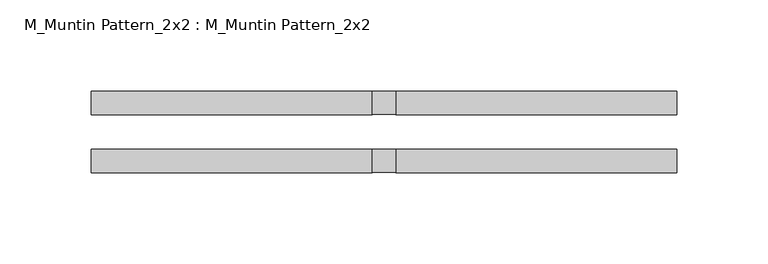
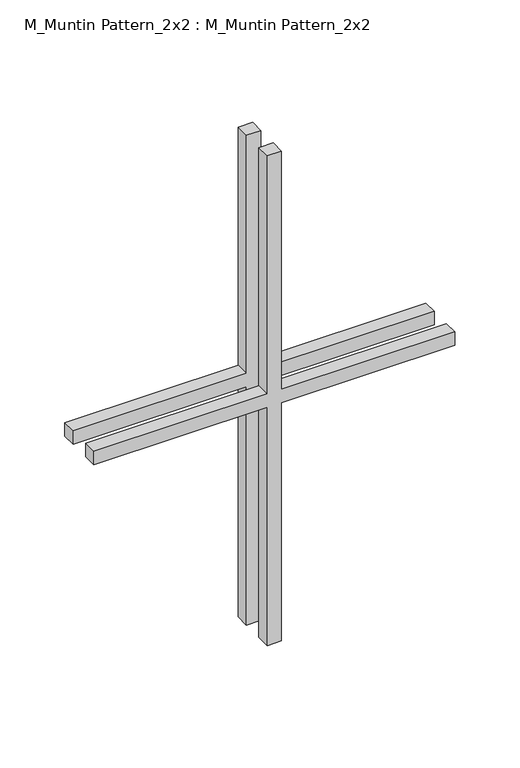
"""IFC4 building model written with IfcOpenShell, lengths in millimetres: proxy geometry, M_Muntin Pattern_2x2 : M_Muntin Pattern_2x2."""

from ifc_helpers import new_model, si_unit, frame, origin, place, context, project, spatial, polyline, outline, extrude, source, transform, mapped, element, save


def m_muntin_pattern_2x2_m_muntin_pattern_2x2_5c9fa27a(model_context):
    return source(origin(), model_context, "Body", "SweptSolid", [
        extrude(outline(polyline([(236.5, -6.35), (236.5, -160.3375), (223.8, -160.3375), (223.8, -6.35), (0.0, -6.35), (0.0, 6.35), (223.8, 6.35), (223.8, 160.3375), (236.5, 160.3375), (236.5, 6.35), (460.3, 6.35), (460.3, -6.35), (236.5, -6.35)])), frame((0.0, 9.525, 0.0), z_axis=(0.0, 1.0, 0.0), x_axis=(0.0, 0.0, 1.0)), (0.0, 0.0, 1.0), 12.7),
        extrude(outline(polyline([(236.5, -6.35), (236.5, -160.3375), (223.8, -160.3375), (223.8, -6.35), (0.0, -6.35), (0.0, 6.35), (223.8, 6.35), (223.8, 160.3375), (236.5, 160.3375), (236.5, 6.35), (460.3, 6.35), (460.3, -6.35), (236.5, -6.35)])), frame((0.0, -22.225, 0.0), z_axis=(0.0, 1.0, 0.0), x_axis=(0.0, 0.0, 1.0)), (0.0, 0.0, 1.0), 12.7),
    ])


if __name__ == "__main__":
    model = new_model("IFC4")
    model_context = context("Model", 3, world=origin())
    ifc_project = project(units=[si_unit("LENGTHUNIT", "METRE", prefix="MILLI")], contexts=[model_context])
    site = spatial("IfcSite", under=ifc_project)
    building = spatial("IfcBuilding", under=site)
    placement = place(None, origin())
    m_muntin_pattern_2x2_m_muntin_pattern_2x2_shape = m_muntin_pattern_2x2_m_muntin_pattern_2x2_5c9fa27a(model_context)
    element("IfcBuildingElementProxy", 1, Name="M_Muntin Pattern_2x2 : M_Muntin Pattern_2x2", ObjectType="M_Muntin Pattern_2x2 : M_Muntin Pattern_2x2", at=placement, inside=building, context=model_context, shape_type="MappedRepresentation", body=[
        mapped(m_muntin_pattern_2x2_m_muntin_pattern_2x2_shape, transform((0.0, 0.0, 0.0), x_axis=(1.0, 0.0, 0.0), y_axis=(0.0, 1.0, 0.0), z_axis=(0.0, 0.0, 1.0))),
    ])
    save(model, "model.ifc")

# Revit data of these elements
# Type "M_Muntin Pattern_2x2 : M_Muntin Pattern_2x2"
#   Width [instance default] = 3' - 11.24409"
#   Thickness = 0' - 0 1/2"
#   Height [instance default] = 3' - 11.24409"
#   Distance = 0' - 0 3/4"
#   Interior Material [instance default] = none
#   Exterior Material [instance default] = none
#   Default Elevation = 0
# Element 1 (IfcBuildingElementProxy, "M_Muntin Pattern_2x2 : M_Muntin Pattern_2x2")
#   Width = 1' - 0 5/8"
#   Height = 1' - 6.12205"
#   Interior Material = Wood - Stained
#   Exterior Material = Clad - White
#   Materials on its faces: "Clad - White", "Wood - Stained"
# Materials
#   "Clad - White": class "Wood", colour RGB 242 242 238, transparency 0, Cost = 0
#   "Wood - Stained": class "Wood", colour RGB 224 178 126, transparency 0, Cost = 0
